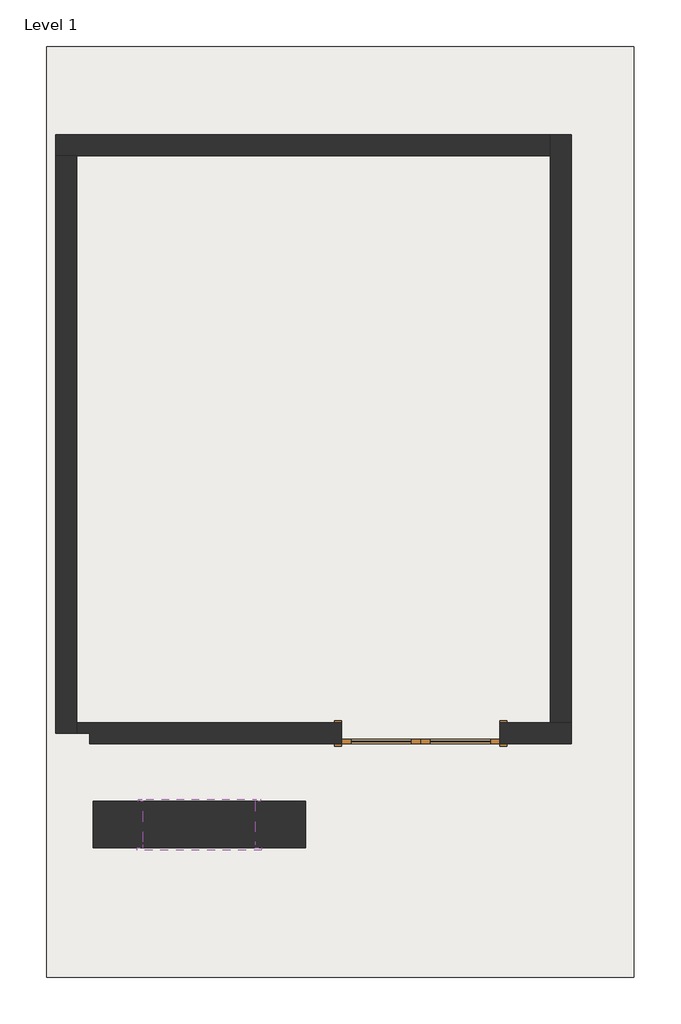
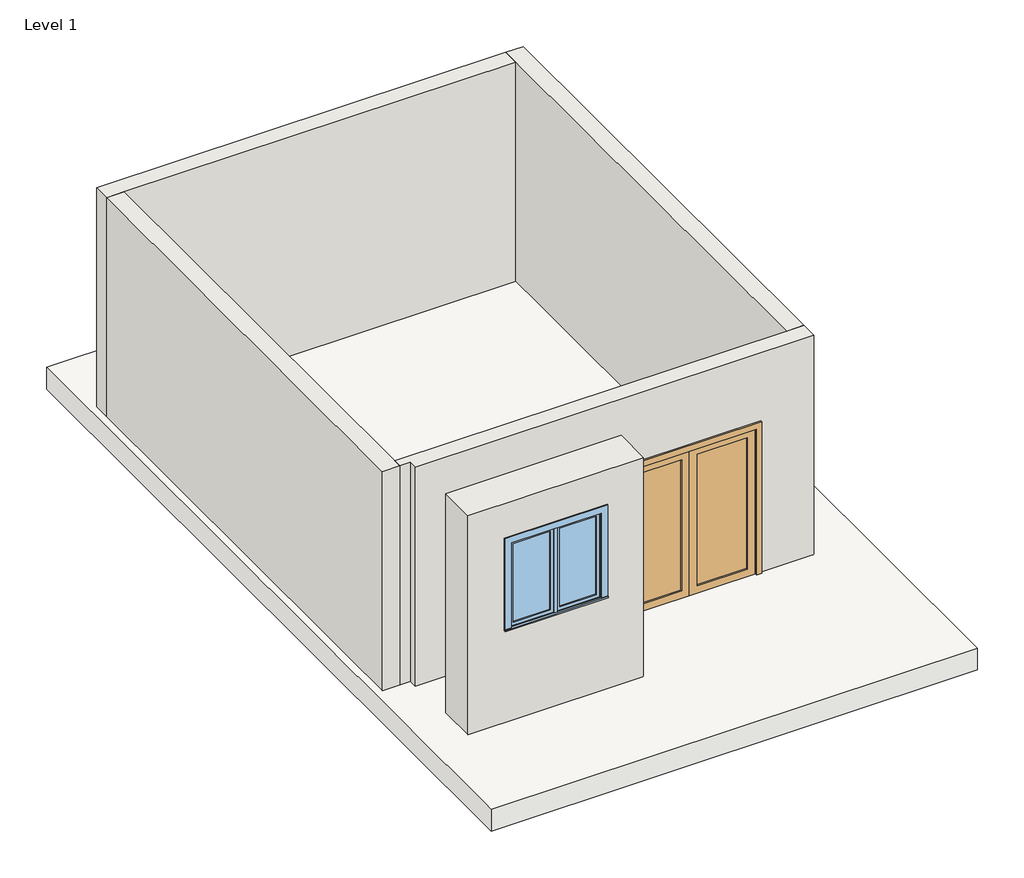
# One storey: 5 walls, 1 door, 1 slab, 1 window.
"""IFC4 building model written with IfcOpenShell, lengths in millimetres."""

from ifc_helpers import new_model, si_unit, frame, origin, place, context, project, spatial, polyline, outline, extrude, faceted_brep, transform, mapped, element, save
from components import door_423d55ee, window_adfa5946

model = new_model("IFC4")

# Units and contexts
model_context = context("Model", 3, world=origin())
ifc_project = project(units=[si_unit("LENGTHUNIT", "METRE", prefix="MILLI")], contexts=[model_context])

# Site, building, storey
site = spatial("IfcSite", under=ifc_project)
building = spatial("IfcBuilding", under=site)
storey = spatial("IfcBuildingStorey", under=building, Name="Level 1", Elevation=0.0)

# Door
placement = place(None, origin())
door_shape = door_423d55ee(model_context)
element("IfcDoor", 1, ObjectType="Door-Double-Glass : 68\" x 80\"", at=placement, inside=storey, context=model_context, shape_type="MappedRepresentation", body=[
    mapped(door_shape, transform((-9230.4306534, 4280.4110237, 0.0), x_axis=(-1.0, 0.0, 0.0), y_axis=(0.0, -1.0, 0.0), z_axis=(0.0, 0.0, 1.0))),
])

# Slab
element("IfcSlab", 2, ObjectType="Generic - 12\"", at=placement, inside=storey, context=model_context, shape_type="SweptSolid", body=[
    extrude(outline(polyline([(-6907.4747935, 11756.2199948), (-6907.4747935, 1621.6199948), (-13308.2747935, 1621.6199948), (-13308.2747935, 11756.2199948), (-6907.4747935, 11756.2199948)])), frame((0.0, 0.0, -304.8), z_axis=(0.0, 0.0, 1.0), x_axis=(1.0, 0.0, 0.0)), (0.0, 0.0, 1.0), 304.8),
])

# Walls
element("IfcWall", 3, ObjectType="Generic - 12\" Masonry", at=placement, inside=storey, context=model_context, shape_type="SweptSolid", body=[
    extrude(outline(polyline([(0.0, -12799.1306534), (0.0, -10487.7306534), (3048.0, -10487.7306534), (3048.0, -12799.1306534), (0.0, -12799.1306534)]), holes=[polyline([(2498.6277554, -12253.0306534), (2498.6277554, -11033.8306534), (1279.4277554, -11033.8306534), (1279.4277554, -12253.0306534), (2498.6277554, -12253.0306534)])]), frame((0.0, 3033.4297737, 0.0), z_axis=(0.0, 1.0, 0.0), x_axis=(0.0, 0.0, 1.0)), (0.0, 0.0, 1.0), 508.0),
])
element("IfcWall", 4, ObjectType="Generic - 9\"", at=placement, inside=storey, context=model_context, shape_type="Brep", body=[
    faceted_brep([(-13205.5306534, 10564.5297737, 0.0), (-12976.9306534, 10564.5297737, 0.0), (-7820.7306534, 10564.5297737, 0.0), (-7820.7306534, 10564.5297737, 3048.0), (-12976.9306534, 10564.5297737, 3048.0), (-13205.5306534, 10564.5297737, 3048.0), (-13205.5306534, 10793.1297737, 0.0), (-13205.5306534, 10793.1297737, 3048.0), (-7820.7306534, 10793.1297737, 3048.0), (-7820.7306534, 10793.1297737, 0.0)], [[[0, 1, 2, 3, 4, 5]], [[6, 7, 8, 9]], [[2, 1, 0, 6, 9]], [[0, 5, 7, 6]], [[7, 5, 4, 3, 8]], [[2, 9, 8, 3]]]),
])
element("IfcWall", 5, ObjectType="Generic - 9\"", at=placement, inside=storey, context=model_context, shape_type="Brep", body=[
    faceted_brep([(-12976.9306534, 4278.0297737, 0.0), (-12976.9306534, 4392.3297737, 0.0), (-12976.9306534, 10564.5297737, 0.0), (-12976.9306534, 10564.5297737, 3048.0), (-12976.9306534, 4392.3297737, 3048.0), (-12976.9306534, 4278.0297737, 3048.0), (-13205.5306534, 4278.0297737, 0.0), (-13205.5306534, 4278.0297737, 3048.0), (-13205.5306534, 10564.5297737, 3048.0), (-13205.5306534, 10564.5297737, 0.0)], [[[0, 1, 2, 3, 4, 5]], [[6, 7, 8, 9]], [[2, 1, 0, 6, 9]], [[2, 9, 8, 3]], [[0, 5, 7, 6]], [[7, 5, 4, 3, 8]]]),
])
element("IfcWall", 6, ObjectType="Generic - 9\"", at=placement, inside=storey, context=model_context, shape_type="Brep", body=[
    faceted_brep([(-10094.0306534, 4392.3297737, 2032.0), (-10094.0306534, 4392.3297737, 0.0), (-12976.9306534, 4392.3297737, 0.0), (-12976.9306534, 4392.3297737, 3048.0), (-7820.7306534, 4392.3297737, 3048.0), (-7592.1306534, 4392.3297737, 3048.0), (-7592.1306534, 4392.3297737, 0.0), (-7820.7306534, 4392.3297737, 0.0), (-8366.8306534, 4392.3297737, 0.0), (-8366.8306534, 4392.3297737, 2032.0), (-12837.2306534, 4163.7297737, 0.0), (-10094.0306534, 4163.7297737, 0.0), (-10094.0306534, 4163.7297737, 2032.0), (-8366.8306534, 4163.7297737, 2032.0), (-8366.8306534, 4163.7297737, 0.0), (-7592.1306534, 4163.7297737, 0.0), (-7592.1306534, 4163.7297737, 3048.0), (-12837.2306534, 4163.7297737, 3048.0), (-12837.2306534, 4278.0297737, 0.0), (-12976.9306534, 4278.0297737, 0.0), (-12976.9306534, 4278.0297737, 3048.0), (-12837.2306534, 4278.0297737, 3048.0)], [[[0, 1, 2, 3, 4, 5, 6, 7, 8, 9]], [[10, 11, 12, 13, 14, 15, 16, 17]], [[2, 1, 11, 10, 18, 19]], [[8, 7, 6, 15, 14]], [[6, 5, 16, 15]], [[16, 5, 4, 3, 20, 21, 17]], [[12, 11, 1, 0]], [[13, 12, 0, 9]], [[14, 13, 9, 8]], [[2, 19, 20, 3]], [[20, 19, 18, 21]], [[21, 18, 10, 17]]]),
])
element("IfcWall", 7, ObjectType="Generic - 9\"", at=placement, inside=storey, context=model_context, shape_type="Brep", body=[
    faceted_brep([(-7820.7306534, 10793.1297737, 0.0), (-7820.7306534, 10564.5297737, 0.0), (-7820.7306534, 4392.3297737, 0.0), (-7820.7306534, 4392.3297737, 3048.0), (-7820.7306534, 10564.5297737, 3048.0), (-7820.7306534, 10793.1297737, 3048.0), (-7592.1306534, 10793.1297737, 0.0), (-7592.1306534, 10793.1297737, 3048.0), (-7592.1306534, 4392.3297737, 3048.0), (-7592.1306534, 4392.3297737, 0.0)], [[[0, 1, 2, 3, 4, 5]], [[6, 7, 8, 9]], [[2, 1, 0, 6, 9]], [[2, 9, 8, 3]], [[0, 5, 7, 6]], [[7, 5, 4, 3, 8]]]),
])

# Window
window_shape = window_adfa5946(model_context)
element("IfcWindow", 8, ObjectType="Casement Dbl with Trim : 48\" x 48\"", at=placement, inside=storey, context=model_context, shape_type="MappedRepresentation", body=[
    mapped(window_shape, transform((-11643.4306534, 3306.4797737, 365.0277554), x_axis=(-1.0, 0.0, 0.0), y_axis=(0.0, -1.0, 0.0), z_axis=(0.0, 0.0, 1.0))),
])

save(model, "model.ifc")

# Revit data of these elements
# Type "Door-Double-Glass : 68\" x 80\""
#   Type Mark = "8"
#   Construction Type Id = "opn-d45"
#   Assembly Code = "C1020"
#   Analytic Construction = "Wood frame, double glass door "
#   W = 2' - 10"
#   Thickness = 0' - 2"
#   Thermal Resistance (R) = 1.8150 (h·ft²·°F)/BTU
#   Swing Angle [instance default] = 90.00°
#   Heat Transfer Coefficient (U) = 0.5510 BTU/(h·ft²·°F)
#   Height = 6' - 8"
#   Bottom Rail = 0' - 4"
#   Top Rail = 0' - 4"
#   Stiles = 0' - 4"
#   Trim Projection = 0' - 1"
#   Trim Width = 0' - 3"
#   Width = 5' - 8"
#   Define Thermal Properties by = 1
#   Glazing = Glass
#   Panel Material = Wood - Birch - Solid Stained Light Low Gloss
#   Trim Material = Paint - Sienna
#   Visual Light Transmittance = 0
#   Solar Heat Gain Coefficient = 0
#   Function = (empty or 0)
#   Wall Closure = (empty or 0)
# Type "Generic - 12\""
#   Assembly Code = "B1010"
#   Function = 0
#   Layers, outside or top first: 1' - 0" no material (function 1)
# Type "Generic - 12\" Masonry"
#   Assembly Code = "B2010"
#   Layers, outside or top first: 1' - 8" "Asphalt Shingle" (function 1)
# Type "Generic - 9\""
#   Assembly Code = "B2010"
#   Layers, outside or top first: 0' - 9" no material (function 1)
# Type "Casement Dbl with Trim : 48\" x 48\""
#   Type Mark = "10"
#   Construction Type Id = "GSP4R"
#   Assembly Code = "B2020100"
#   Analytic Construction = "1/8 in Pilkington single glazing"
#   Visual Light Transmittance = 0.9
#   Solar Heat Gain Coefficient = 0.78
#   Heat Transfer Coefficient (U) = 0.6496 BTU/(h·ft²·°F)
#   Height = 4' - 0"
#   Default Sill Height = 3' - 0"
#   Trim Projection - Ext. = 0' - 0 1/2"
#   Trim Projection - Int. = 0' - 0 3/4"
#   Trim Width - Exterior = 0' - 3 1/2"
#   Trim Width - Interior = 0' - 3 1/2"
#   Width = 4' - 0"
#   Window Inset = 0' - 0 3/4"
#   Define Thermal Properties by = 1
#   Glass Pane Material = Glass
#   Sash Material = Roofing, EPDM Membrane
#   Trim Exterior Material = Roofing, EPDM Membrane
#   Trim Interior Material = Trim
#   Wall Closure = (empty or 0)
# Element 1 (IfcDoor, "Door-Double-Glass : 68\" x 80\"")
#   Swing Angle = 90.00°
#   Phase Created = New Construction
#   Materials on its faces: "Wood - Birch - Solid Stained Light Low Gloss", "Paint - Sienna", "Glass"
# Element 2 (IfcSlab, "Generic - 12\"")
#   Height Offset From Level = 0' - 0"
#   Phase Created = New Construction
#   Materials on its faces: "Default Floor"
# Element 3 (IfcWall, "Generic - 12\" Masonry")
#   Top Offset = 0' - 0"
#   Base Offset = 0' - 0"
#   Unconnected Height = 10' - 0"
#   wall height = 10' - 0"
#   Phase Created = New Construction
#   Base Constraint = Level 1
#   Materials on its faces: "Asphalt Shingle"
# Elements 4, 5, 6, 7 (IfcWall, "Generic - 9\"")
#   Top Offset = 0' - 0"
#   Base Offset = 0' - 0"
#   Unconnected Height = 12' - 0"
#   wall height = 12' - 0"
#   Phase Created = New Construction
#   Base Constraint = Level 1
#   Materials on its faces: "Default Wall"
# Element 8 (IfcWindow, "Casement Dbl with Trim : 48\" x 48\"")
#   Mark = "5"
#   Phase Created = New Construction
#   Materials on its faces: "Roofing, EPDM Membrane", "Glass", "Trim"
# Materials
#   "Glass": class "Glass", colour RGB 0 128 192, transparency 0.75, Description = "Soda Lime Glass", Cost = 0
#   "Wood - Birch - Solid Stained Light Low Gloss": class "Wood", colour RGB 210 159 95, transparency 0, Cost = 0
#   "Paint - Sienna": colour RGB 118 70 51, transparency 0, Cost = 0
#   "Asphalt Shingle": class "Generic", colour RGB 155 155 155, transparency 0, Description = "Asphalt roofing shingle", Cost = 0
#   "Roofing, EPDM Membrane": class "Generic", colour RGB 127 127 127, transparency 0, Description = "EPDM roof membrane", Cost = 0
#   "Trim": class "Wood", colour RGB 224 178 126, transparency 0
#   "Default Floor": colour RGB 128 128 128, transparency 0
#   "Default Wall": colour RGB 128 128 128, transparency 0
